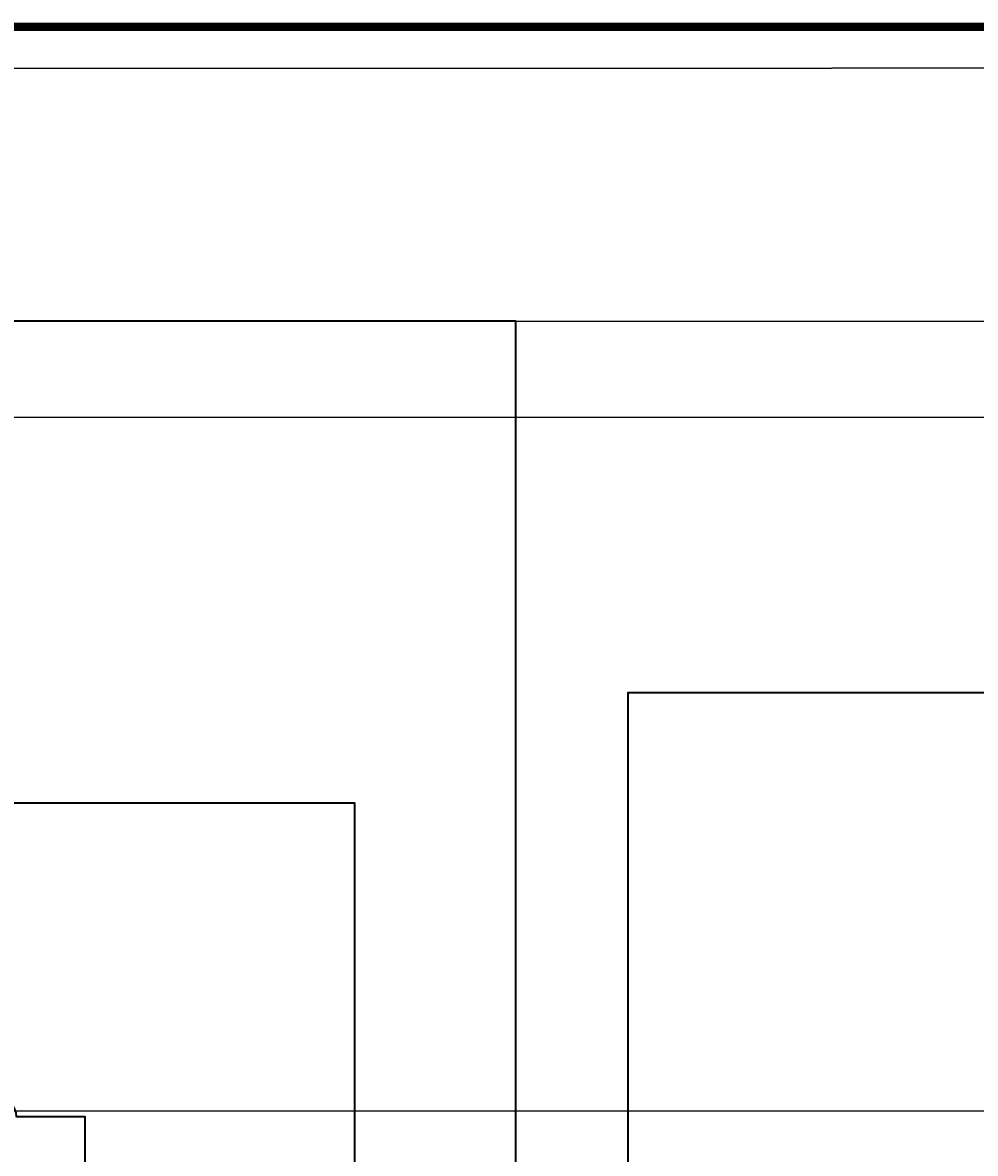
# Model space of a CAD drawing. Units: millimetres. Extents: x 353872 to 441597, y 126154 to 187356.
# Tile 19 of 28: x 382257 to 399262, y 167178 to 187356. Entities that reach past the tile are written whole.
import ezdxf

# ---------------------------------------------------------------- set-up
doc = ezdxf.new("R2010")
doc.units = ezdxf.units.MM
for name, color, linetype, lineweight in [('A-ANNO-DIMS', 2, 'Continuous', 18), ('P-ANNO-TTLB', 7, 'Continuous', 25), ('P-PIPE', 3, 'Continuous', 35)]:
    doc.layers.add(name, color=color, linetype=linetype, lineweight=lineweight)
doc.styles.get("Standard").update_dxf_attribs({"font": 'arial.ttf'})
doc.dimstyles.get("Standard").update_dxf_attribs({"dimtxt": 0.18, "dimasz": 0.18, "dimexe": 0.18, "dimexo": 0.0625, "dimgap": 0.09, "dimtad": 0, "dimtih": 1, "dimtoh": 1, "dimdec": 4, "dimzin": 0, "dimdsep": 46, "dimtxsty": 'Standard', "dimcen": 0.09, "dimadec": 0, "dimazin": 0, "dimtfac": 1, "dimtdec": 4, "dimtofl": 0, "dimtmove": 0, "dimatfit": 3, "dimfxl": 1, "dimtolj": 1, "dimtzin": 0, "dimarcsym": 0})

# ---------------------------------------------------------------- blocks, each defined once
blk = doc.blocks.new('*D24')
at = {"layer": 'A-ANNO-DIMS', "color": 0, "lineweight": -2, "transparency": 16777216}
for p, q in [((360737, 182546), (360737, 186546)), ((360737, 186546), (396698, 186546)), ((432661, 186546), (396699, 186546)), ((432661, 177114), (432661, 186546))]:
    blk.add_line(p, q, dxfattribs=at)
at = {"layer": 'A-ANNO-DIMS', "color": 0, "transparency": 16777216}
for points in [[(360737, 186546), (360737, 186546), (360737, 186546)], [(432661, 186546), (432661, 186546), (432661, 186546)]]:
    blk.add_solid(points, dxfattribs=at)
at = {"layer": 'Defpoints', "color": 0, "transparency": 16777216}
for p in [(432661, 186546), (360737, 182546), (432661, 177114)]:
    blk.add_point(p, dxfattribs=at)
at = {"layer": 'A-ANNO-DIMS', "color": 0, "transparency": 16777216, "insert": (396699, 186546), "char_height": 0.18, "attachment_point": 5}
blk.add_mtext('\\A1;71924', dxfattribs=at)
blk = doc.blocks.new('*D28')
at = {"layer": 'A-ANNO-DIMS', "color": 0, "lineweight": -2, "transparency": 16777216}
for p, q in [((366977, 182028), (440591, 182028)), ((440591, 182028), (440591, 181171)), ((440591, 180314), (440591, 181171)), ((366977, 180314), (440591, 180314))]:
    blk.add_line(p, q, dxfattribs=at)
at = {"layer": 'A-ANNO-DIMS', "color": 0, "transparency": 16777216}
for points in [[(440591, 182028), (440591, 182028), (440591, 182028)], [(440591, 180314), (440591, 180314), (440591, 180314)]]:
    blk.add_solid(points, dxfattribs=at)
at = {"layer": 'Defpoints', "color": 0, "transparency": 16777216}
for p in [(366977, 182028), (366977, 180314), (440591, 180314)]:
    blk.add_point(p, dxfattribs=at)
at = {"layer": 'A-ANNO-DIMS', "color": 0, "transparency": 16777216, "insert": (440591, 181171), "char_height": 0.18, "attachment_point": 5}
blk.add_mtext('\\A1;1714.5', dxfattribs=at)
blk = doc.blocks.new('*D34')
at = {"layer": 'A-ANNO-DIMS', "color": 0, "lineweight": -2, "transparency": 16777216}
for p, q in [((399457, 167930), (356736, 167930)), ((356737, 167930), (356737, 163994)), ((356737, 160058), (356737, 163994)), ((399457, 160058), (356736, 160058))]:
    blk.add_line(p, q, dxfattribs=at)
at = {"layer": 'A-ANNO-DIMS', "color": 0, "transparency": 16777216}
for points in [[(356737, 167930), (356737, 167930), (356737, 167930)], [(356737, 160058), (356737, 160058), (356737, 160058)]]:
    blk.add_solid(points, dxfattribs=at)
at = {"layer": 'Defpoints', "color": 0, "transparency": 16777216}
for p in [(399457, 167930), (356737, 160058), (399457, 160058)]:
    blk.add_point(p, dxfattribs=at)
at = {"layer": 'A-ANNO-DIMS', "color": 0, "transparency": 16777216, "insert": (356737, 163994), "char_height": 0.18, "attachment_point": 5}
blk.add_mtext('\\A1;7872', dxfattribs=at)

msp = doc.modelspace()

# ---------------------------------------------------------------- linework, layer by layer
at = {"layer": 'P-ANNO-TTLB', "const_width": 152.43}
msp.add_lwpolyline([(353948.03, 187280.05), (353948.03, 126916.34), (440835.19, 126916.34), (440835.19, 187280.05)], close=True, dxfattribs=at)
at = {"layer": 'P-PIPE'}
for points in [[(391060.3, 150079.91), (391060.3, 182028.44), (390103.2, 182028.44), (366976.76, 182028.44)], [(393066.71, 149319.73), (393066.71, 175399.89), (426420.76, 175399.89)], [(366976.76, 173434.34), (386613.67, 173434.34), (388181.19, 173434.34), (388181.19, 163303.71)]]:
    msp.add_lwpolyline(points, dxfattribs=at)
msp.add_lwpolyline([(388213.21, 147045.52), (383375.2, 147045.17), (383375.2, 147045.17), (383375.2, 149602.24), (383375.2, 167832.6), (382147.59, 167832.6, 1), (381458.98, 167832.6), (380124.81, 167832.6, 1), (379436.2, 167832.6), (368453.37, 167832.6)], format="xyb", dxfattribs=at)

# ---------------------------------------------------------------- dimensions: what is measured, and where the dimension line sits
at = {"layer": 'A-ANNO-DIMS'}
dim = msp.add_linear_dim(base=(432660.97, 186546.05), p1=(360736.55, 182546.05), p2=(432660.97, 177114.41), dimstyle='Standard', override={"dimdec": 0, "dimlfac": 1, "dimrnd": 0, "dimzin": 0, "dimdsep": 46, "dimlunit": 2}, dxfattribs=at)
dim.commit()
dim.dimension.update_dxf_attribs({"geometry": '*D24', "text_midpoint": (396698.76, 186546.05)})
for base, p1, p2, override, picture, middle in [((440591, 180313.91), (366976.76, 182028.44), (366976.76, 180313.91), {"dimdec": 1, "dimlfac": 1, "dimrnd": 0, "dimzin": 0, "dimdsep": 46, "dimlunit": 2}, '*D28', (440591, 181171.18)), ((356736.55, 160058.19), (399457.15, 167929.97), (399457.15, 160058.19), {"dimdec": 0, "dimlfac": 1, "dimrnd": 0, "dimzin": 0, "dimdsep": 46, "dimlunit": 2}, '*D34', (356736.55, 163994.08))]:
    dim = msp.add_linear_dim(base=base, p1=p1, p2=p2, angle=90, dimstyle='Standard', override=override, dxfattribs=at)
    dim.commit()
    dim.dimension.update_dxf_attribs({"geometry": picture, "text_midpoint": middle})

doc.saveas('drawing.dxf')
